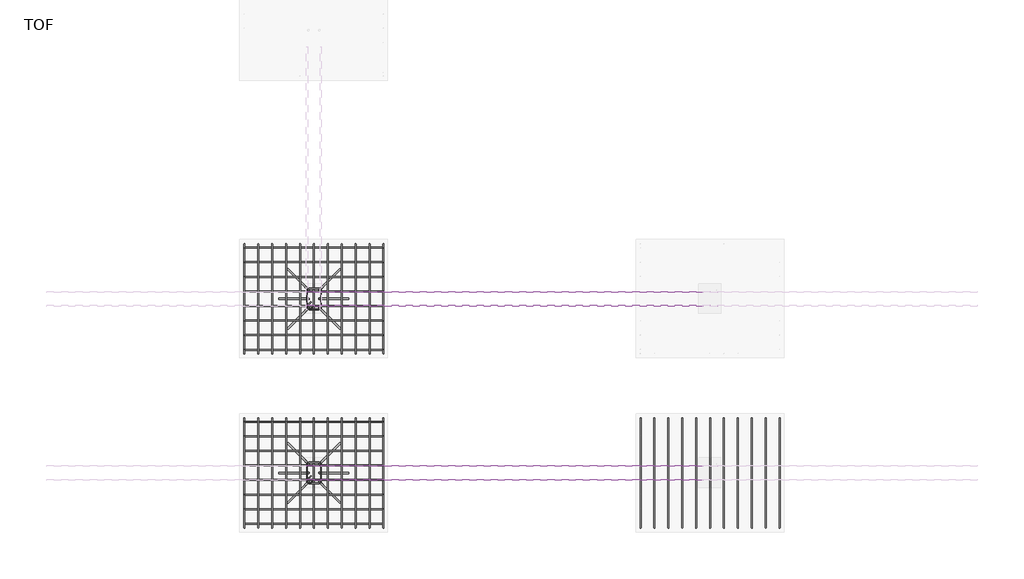
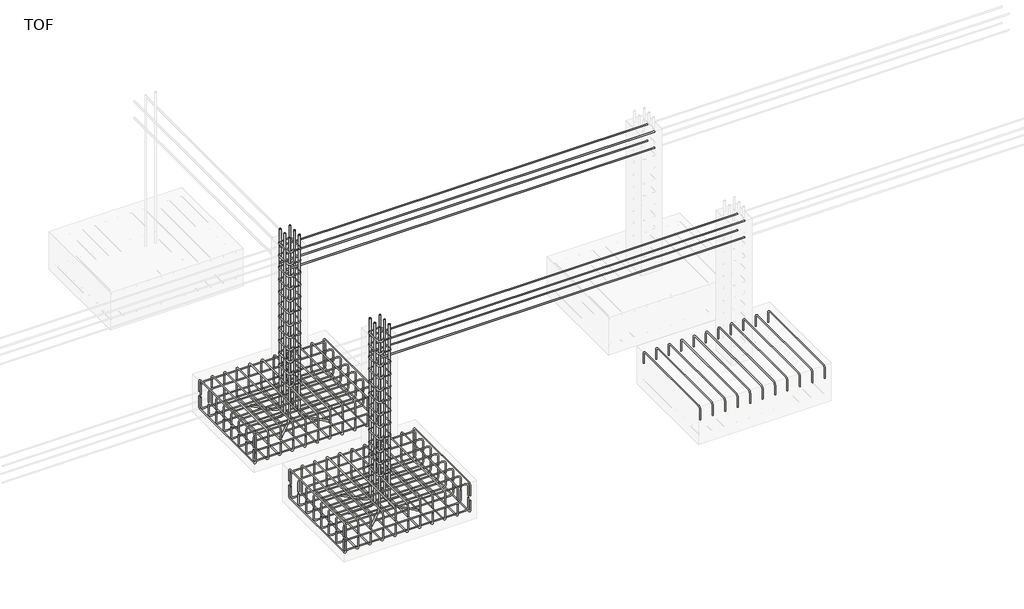
# One storey, part 4 of 10: 31 reinforcing bars.
"""IFC4 building model written with IfcOpenShell, lengths in millimetres."""

from ifc_helpers import new_model, si_unit, point, frame, origin, place, context, project, spatial, polyline, circle_curve, trimmed, segment, composite_curve, source, transform, mapped, element, save
from ifc_brep_helpers import swept_disk

model = new_model("IFC4")

# Units and contexts
model_context = context("Model", 3, world=origin())
ifc_project = project(units=[si_unit("LENGTHUNIT", "METRE", prefix="MILLI")], contexts=[model_context])

# Site, building, storey
site = spatial("IfcSite", under=ifc_project)
building = spatial("IfcBuilding", under=site)
storey = spatial("IfcBuildingStorey", under=building, Name="TOF", Elevation=-1828.8)

# Reinforcing bars
placement = place(None, origin())
reinforcing_bar_shape = source(origin(), model_context, "Body", "SolidModel", [
    swept_disk(composite_curve([segment(polyline([(2315.2782143, -14539.6267376, -2018.8), (2315.2782143, -14539.6267376, -1908.8)]), True, "CONTINUOUS"), segment(trimmed(circle_curve(frame((2315.2782143, -14574.6267376, -1908.8), z_axis=(1.0, 0.0, 0.0), x_axis=(0.0, 35.0, 0.0)), 35.0), [point((2315.2782143, -14539.6267376, -1908.8))], [point((2315.2782143, -14574.6267376, -1873.8))], True, "CARTESIAN"), True, "CONTINUOUS"), segment(polyline([(2315.2782143, -14574.6267376, -1873.8), (2315.2782143, -15614.6267376, -1873.8)]), True, "CONTINUOUS"), segment(trimmed(circle_curve(frame((2315.2782143, -15614.6267376, -1908.8), z_axis=(1.0, 0.0, 0.0), x_axis=(0.0, 0.0, 35.0)), 35.0), [point((2315.2782143, -15614.6267376, -1873.8))], [point((2315.2782143, -15649.6267376, -1908.8))], True, "CARTESIAN"), True, "CONTINUOUS"), segment(polyline([(2315.2782143, -15649.6267376, -1908.8), (2315.2782143, -15649.6267376, -2018.8)]), True, "CONTINUOUS")], self_intersect=False), 5.0),
])
element("IfcReinforcingBar", 1, at=placement, inside=storey, context=model_context, shape_type="MappedRepresentation", body=[
    mapped(reinforcing_bar_shape, transform((0.0, 0.0, 0.0), x_axis=(1.0, 0.0, 0.0), y_axis=(0.0, 1.0, 0.0), z_axis=(0.0, 0.0, 1.0))),
    mapped(reinforcing_bar_shape, transform((-141.0, 0.0, 0.0), x_axis=(1.0, 0.0, 0.0), y_axis=(0.0, 1.0, 0.0), z_axis=(0.0, 0.0, 1.0))),
    mapped(reinforcing_bar_shape, transform((-282.0, 0.0, 0.0), x_axis=(1.0, 0.0, 0.0), y_axis=(0.0, 1.0, 0.0), z_axis=(0.0, 0.0, 1.0))),
    mapped(reinforcing_bar_shape, transform((-423.0, 0.0, 0.0), x_axis=(1.0, 0.0, 0.0), y_axis=(0.0, 1.0, 0.0), z_axis=(0.0, 0.0, 1.0))),
    mapped(reinforcing_bar_shape, transform((-564.0, 0.0, 0.0), x_axis=(1.0, 0.0, 0.0), y_axis=(0.0, 1.0, 0.0), z_axis=(0.0, 0.0, 1.0))),
    mapped(reinforcing_bar_shape, transform((-705.0, 0.0, 0.0), x_axis=(1.0, 0.0, 0.0), y_axis=(0.0, 1.0, 0.0), z_axis=(0.0, 0.0, 1.0))),
    mapped(reinforcing_bar_shape, transform((-846.0, 0.0, 0.0), x_axis=(1.0, 0.0, 0.0), y_axis=(0.0, 1.0, 0.0), z_axis=(0.0, 0.0, 1.0))),
    mapped(reinforcing_bar_shape, transform((-987.0, 0.0, 0.0), x_axis=(1.0, 0.0, 0.0), y_axis=(0.0, 1.0, 0.0), z_axis=(0.0, 0.0, 1.0))),
    mapped(reinforcing_bar_shape, transform((-1128.0, 0.0, 0.0), x_axis=(1.0, 0.0, 0.0), y_axis=(0.0, 1.0, 0.0), z_axis=(0.0, 0.0, 1.0))),
    mapped(reinforcing_bar_shape, transform((-1269.0, 0.0, 0.0), x_axis=(1.0, 0.0, 0.0), y_axis=(0.0, 1.0, 0.0), z_axis=(0.0, 0.0, 1.0))),
    mapped(reinforcing_bar_shape, transform((-1410.0, 0.0, 0.0), x_axis=(1.0, 0.0, 0.0), y_axis=(0.0, 1.0, 0.0), z_axis=(0.0, 0.0, 1.0))),
])
reinforcing_bar_2_shape = source(origin(), model_context, "Body", "SolidModel", [
    swept_disk(composite_curve([segment(polyline([(2315.2782143, -15649.6267376, -2077.5233378), (2315.2782143, -15649.6267376, -2187.5233378)]), True, "CONTINUOUS"), segment(trimmed(circle_curve(frame((2315.2782143, -15614.6267376, -2187.5233378), z_axis=(1.0, 0.0, 0.0), x_axis=(0.0, -35.0, 0.0)), 35.0), [point((2315.2782143, -15649.6267376, -2187.5233378))], [point((2315.2782143, -15614.6267376, -2222.5233378))], True, "CARTESIAN"), True, "CONTINUOUS"), segment(polyline([(2315.2782143, -15614.6267376, -2222.5233378), (2315.2782143, -14574.6267376, -2222.5233378)]), True, "CONTINUOUS"), segment(trimmed(circle_curve(frame((2315.2782143, -14574.6267376, -2187.5233378), z_axis=(1.0, 0.0, 0.0), x_axis=(0.0, 0.0, -35.0)), 35.0), [point((2315.2782143, -14574.6267376, -2222.5233378))], [point((2315.2782143, -14539.6267376, -2187.5233378))], True, "CARTESIAN"), True, "CONTINUOUS"), segment(polyline([(2315.2782143, -14539.6267376, -2187.5233378), (2315.2782143, -14539.6267376, -2077.5233378)]), True, "CONTINUOUS")], self_intersect=False), 5.0),
])
element("IfcReinforcingBar", 2, at=placement, inside=storey, context=model_context, shape_type="MappedRepresentation", body=[
    mapped(reinforcing_bar_2_shape, transform((0.0, 0.0, 0.0), x_axis=(1.0, 0.0, 0.0), y_axis=(0.0, 1.0, 0.0), z_axis=(0.0, 0.0, 1.0))),
    mapped(reinforcing_bar_2_shape, transform((-141.0, 0.0, 0.0), x_axis=(1.0, 0.0, 0.0), y_axis=(0.0, 1.0, 0.0), z_axis=(0.0, 0.0, 1.0))),
    mapped(reinforcing_bar_2_shape, transform((-282.0, 0.0, 0.0), x_axis=(1.0, 0.0, 0.0), y_axis=(0.0, 1.0, 0.0), z_axis=(0.0, 0.0, 1.0))),
    mapped(reinforcing_bar_2_shape, transform((-423.0, 0.0, 0.0), x_axis=(1.0, 0.0, 0.0), y_axis=(0.0, 1.0, 0.0), z_axis=(0.0, 0.0, 1.0))),
    mapped(reinforcing_bar_2_shape, transform((-564.0, 0.0, 0.0), x_axis=(1.0, 0.0, 0.0), y_axis=(0.0, 1.0, 0.0), z_axis=(0.0, 0.0, 1.0))),
    mapped(reinforcing_bar_2_shape, transform((-705.0, 0.0, 0.0), x_axis=(1.0, 0.0, 0.0), y_axis=(0.0, 1.0, 0.0), z_axis=(0.0, 0.0, 1.0))),
    mapped(reinforcing_bar_2_shape, transform((-846.0, 0.0, 0.0), x_axis=(1.0, 0.0, 0.0), y_axis=(0.0, 1.0, 0.0), z_axis=(0.0, 0.0, 1.0))),
    mapped(reinforcing_bar_2_shape, transform((-987.0, 0.0, 0.0), x_axis=(1.0, 0.0, 0.0), y_axis=(0.0, 1.0, 0.0), z_axis=(0.0, 0.0, 1.0))),
    mapped(reinforcing_bar_2_shape, transform((-1128.0, 0.0, 0.0), x_axis=(1.0, 0.0, 0.0), y_axis=(0.0, 1.0, 0.0), z_axis=(0.0, 0.0, 1.0))),
    mapped(reinforcing_bar_2_shape, transform((-1269.0, 0.0, 0.0), x_axis=(1.0, 0.0, 0.0), y_axis=(0.0, 1.0, 0.0), z_axis=(0.0, 0.0, 1.0))),
    mapped(reinforcing_bar_2_shape, transform((-1410.0, 0.0, 0.0), x_axis=(1.0, 0.0, 0.0), y_axis=(0.0, 1.0, 0.0), z_axis=(0.0, 0.0, 1.0))),
])
reinforcing_bar_3_shape = source(origin(), model_context, "Body", "SolidModel", [
    swept_disk(composite_curve([segment(polyline([(2315.2782143, -14574.6861459, -2066.1776706), (2315.2782143, -14574.6861459, -2176.1776706)]), True, "CONTINUOUS"), segment(trimmed(circle_curve(frame((2280.2782143, -14574.6861459, -2176.1776706), z_axis=(0.0, 1.0, 0.0), x_axis=(35.0, 0.0, 0.0)), 35.0), [point((2315.2782143, -14574.6861459, -2176.1776706))], [point((2280.2782143, -14574.6861459, -2211.1776706))], True, "CARTESIAN"), True, "CONTINUOUS"), segment(polyline([(2280.2782143, -14574.6861459, -2211.1776706), (940.2782143, -14574.6861459, -2211.1776706)]), True, "CONTINUOUS"), segment(trimmed(circle_curve(frame((940.2782143, -14574.6861459, -2176.1776706), z_axis=(0.0, 1.0, 0.0), x_axis=(0.0, 0.0, -35.0)), 35.0), [point((940.2782143, -14574.6861459, -2211.1776706))], [point((905.2782143, -14574.6861459, -2176.1776706))], True, "CARTESIAN"), True, "CONTINUOUS"), segment(polyline([(905.2782143, -14574.6861459, -2176.1776706), (905.2782143, -14574.6861459, -2066.1776706)]), True, "CONTINUOUS")], self_intersect=False), 5.0),
])
element("IfcReinforcingBar", 3, at=placement, inside=storey, context=model_context, shape_type="MappedRepresentation", body=[
    mapped(reinforcing_bar_3_shape, transform((0.0, 0.0, 0.0), x_axis=(1.0, 0.0, 0.0), y_axis=(0.0, 1.0, 0.0), z_axis=(0.0, 0.0, 1.0))),
    mapped(reinforcing_bar_3_shape, transform((0.0, -148.0321606, 0.0), x_axis=(1.0, 0.0, 0.0), y_axis=(0.0, 1.0, 0.0), z_axis=(0.0, 0.0, 1.0))),
    mapped(reinforcing_bar_3_shape, transform((0.0, -296.0643211, 0.0), x_axis=(1.0, 0.0, 0.0), y_axis=(0.0, 1.0, 0.0), z_axis=(0.0, 0.0, 1.0))),
    mapped(reinforcing_bar_3_shape, transform((0.0, -444.0964817, 0.0), x_axis=(1.0, 0.0, 0.0), y_axis=(0.0, 1.0, 0.0), z_axis=(0.0, 0.0, 1.0))),
    mapped(reinforcing_bar_3_shape, transform((0.0, -592.1286423, 0.0), x_axis=(1.0, 0.0, 0.0), y_axis=(0.0, 1.0, 0.0), z_axis=(0.0, 0.0, 1.0))),
    mapped(reinforcing_bar_3_shape, transform((0.0, -740.1608029, 0.0), x_axis=(1.0, 0.0, 0.0), y_axis=(0.0, 1.0, 0.0), z_axis=(0.0, 0.0, 1.0))),
    mapped(reinforcing_bar_3_shape, transform((0.0, -888.1929634, 0.0), x_axis=(1.0, 0.0, 0.0), y_axis=(0.0, 1.0, 0.0), z_axis=(0.0, 0.0, 1.0))),
    mapped(reinforcing_bar_3_shape, transform((0.0, -1036.225124, 0.0), x_axis=(1.0, 0.0, 0.0), y_axis=(0.0, 1.0, 0.0), z_axis=(0.0, 0.0, 1.0))),
])
reinforcing_bar_4_shape = source(origin(), model_context, "Body", "SolidModel", [
    swept_disk(composite_curve([segment(polyline([(2315.2782143, -15610.9112699, -2039.256778), (2315.2782143, -15610.9112699, -1929.256778)]), True, "CONTINUOUS"), segment(trimmed(circle_curve(frame((2280.2782143, -15610.9112699, -1929.256778), z_axis=(0.0, -1.0, 0.0), x_axis=(35.0, 0.0, 0.0)), 35.0), [point((2315.2782143, -15610.9112699, -1929.256778))], [point((2280.2782143, -15610.9112699, -1894.256778))], True, "CARTESIAN"), True, "CONTINUOUS"), segment(polyline([(2280.2782143, -15610.9112699, -1894.256778), (940.2782143, -15610.9112699, -1894.256778)]), True, "CONTINUOUS"), segment(trimmed(circle_curve(frame((940.2782143, -15610.9112699, -1929.256778), z_axis=(0.0, -1.0, 0.0), x_axis=(0.0, 0.0, 35.0)), 35.0), [point((940.2782143, -15610.9112699, -1894.256778))], [point((905.2782143, -15610.9112699, -1929.256778))], True, "CARTESIAN"), True, "CONTINUOUS"), segment(polyline([(905.2782143, -15610.9112699, -1929.256778), (905.2782143, -15610.9112699, -2039.256778)]), True, "CONTINUOUS")], self_intersect=False), 5.0),
])
element("IfcReinforcingBar", 4, at=placement, inside=storey, context=model_context, shape_type="MappedRepresentation", body=[
    mapped(reinforcing_bar_4_shape, transform((0.0, 0.0, 0.0), x_axis=(1.0, 0.0, 0.0), y_axis=(0.0, 1.0, 0.0), z_axis=(0.0, 0.0, 1.0))),
    mapped(reinforcing_bar_4_shape, transform((0.0, 148.0321606, 0.0), x_axis=(1.0, 0.0, 0.0), y_axis=(0.0, 1.0, 0.0), z_axis=(0.0, 0.0, 1.0))),
    mapped(reinforcing_bar_4_shape, transform((0.0, 296.0643211, 0.0), x_axis=(1.0, 0.0, 0.0), y_axis=(0.0, 1.0, 0.0), z_axis=(0.0, 0.0, 1.0))),
    mapped(reinforcing_bar_4_shape, transform((0.0, 444.0964817, 0.0), x_axis=(1.0, 0.0, 0.0), y_axis=(0.0, 1.0, 0.0), z_axis=(0.0, 0.0, 1.0))),
    mapped(reinforcing_bar_4_shape, transform((0.0, 592.1286423, 0.0), x_axis=(1.0, 0.0, 0.0), y_axis=(0.0, 1.0, 0.0), z_axis=(0.0, 0.0, 1.0))),
    mapped(reinforcing_bar_4_shape, transform((0.0, 740.1608029, 0.0), x_axis=(1.0, 0.0, 0.0), y_axis=(0.0, 1.0, 0.0), z_axis=(0.0, 0.0, 1.0))),
    mapped(reinforcing_bar_4_shape, transform((0.0, 888.1929634, 0.0), x_axis=(1.0, 0.0, 0.0), y_axis=(0.0, 1.0, 0.0), z_axis=(0.0, 0.0, 1.0))),
    mapped(reinforcing_bar_4_shape, transform((0.0, 1036.225124, 0.0), x_axis=(1.0, 0.0, 0.0), y_axis=(0.0, 1.0, 0.0), z_axis=(0.0, 0.0, 1.0))),
])
reinforcing_bar_5_shape = source(origin(), model_context, "Body", "SolidModel", [
    swept_disk(composite_curve([segment(polyline([(6330.2782143, -14539.6267376, -2018.8), (6330.2782143, -14539.6267376, -1908.8)]), True, "CONTINUOUS"), segment(trimmed(circle_curve(frame((6330.2782143, -14574.6267376, -1908.8), z_axis=(1.0, 0.0, 0.0), x_axis=(0.0, 35.0, 0.0)), 35.0), [point((6330.2782143, -14539.6267376, -1908.8))], [point((6330.2782143, -14574.6267376, -1873.8))], True, "CARTESIAN"), True, "CONTINUOUS"), segment(polyline([(6330.2782143, -14574.6267376, -1873.8), (6330.2782143, -15614.6267376, -1873.8)]), True, "CONTINUOUS"), segment(trimmed(circle_curve(frame((6330.2782143, -15614.6267376, -1908.8), z_axis=(1.0, 0.0, 0.0), x_axis=(0.0, 0.0, 35.0)), 35.0), [point((6330.2782143, -15614.6267376, -1873.8))], [point((6330.2782143, -15649.6267376, -1908.8))], True, "CARTESIAN"), True, "CONTINUOUS"), segment(polyline([(6330.2782143, -15649.6267376, -1908.8), (6330.2782143, -15649.6267376, -2018.8)]), True, "CONTINUOUS")], self_intersect=False), 5.0),
])
element("IfcReinforcingBar", 5, at=placement, inside=storey, context=model_context, shape_type="MappedRepresentation", body=[
    mapped(reinforcing_bar_5_shape, transform((0.0, 0.0, 0.0), x_axis=(1.0, 0.0, 0.0), y_axis=(0.0, 1.0, 0.0), z_axis=(0.0, 0.0, 1.0))),
    mapped(reinforcing_bar_5_shape, transform((-141.0, 0.0, 0.0), x_axis=(1.0, 0.0, 0.0), y_axis=(0.0, 1.0, 0.0), z_axis=(0.0, 0.0, 1.0))),
    mapped(reinforcing_bar_5_shape, transform((-282.0, 0.0, 0.0), x_axis=(1.0, 0.0, 0.0), y_axis=(0.0, 1.0, 0.0), z_axis=(0.0, 0.0, 1.0))),
    mapped(reinforcing_bar_5_shape, transform((-423.0, 0.0, 0.0), x_axis=(1.0, 0.0, 0.0), y_axis=(0.0, 1.0, 0.0), z_axis=(0.0, 0.0, 1.0))),
    mapped(reinforcing_bar_5_shape, transform((-564.0, 0.0, 0.0), x_axis=(1.0, 0.0, 0.0), y_axis=(0.0, 1.0, 0.0), z_axis=(0.0, 0.0, 1.0))),
    mapped(reinforcing_bar_5_shape, transform((-705.0, 0.0, 0.0), x_axis=(1.0, 0.0, 0.0), y_axis=(0.0, 1.0, 0.0), z_axis=(0.0, 0.0, 1.0))),
    mapped(reinforcing_bar_5_shape, transform((-846.0, 0.0, 0.0), x_axis=(1.0, 0.0, 0.0), y_axis=(0.0, 1.0, 0.0), z_axis=(0.0, 0.0, 1.0))),
    mapped(reinforcing_bar_5_shape, transform((-987.0, 0.0, 0.0), x_axis=(1.0, 0.0, 0.0), y_axis=(0.0, 1.0, 0.0), z_axis=(0.0, 0.0, 1.0))),
    mapped(reinforcing_bar_5_shape, transform((-1128.0, 0.0, 0.0), x_axis=(1.0, 0.0, 0.0), y_axis=(0.0, 1.0, 0.0), z_axis=(0.0, 0.0, 1.0))),
    mapped(reinforcing_bar_5_shape, transform((-1269.0, 0.0, 0.0), x_axis=(1.0, 0.0, 0.0), y_axis=(0.0, 1.0, 0.0), z_axis=(0.0, 0.0, 1.0))),
    mapped(reinforcing_bar_5_shape, transform((-1410.0, 0.0, 0.0), x_axis=(1.0, 0.0, 0.0), y_axis=(0.0, 1.0, 0.0), z_axis=(0.0, 0.0, 1.0))),
])
reinforcing_bar_6_shape = source(origin(), model_context, "Body", "SolidModel", [
    swept_disk(composite_curve([segment(polyline([(2315.2782143, -12774.6267376, -2018.8), (2315.2782143, -12774.6267376, -1908.8)]), True, "CONTINUOUS"), segment(trimmed(circle_curve(frame((2315.2782143, -12809.6267376, -1908.8), z_axis=(1.0, 0.0, 0.0), x_axis=(0.0, 35.0, 0.0)), 35.0), [point((2315.2782143, -12774.6267376, -1908.8))], [point((2315.2782143, -12809.6267376, -1873.8))], True, "CARTESIAN"), True, "CONTINUOUS"), segment(polyline([(2315.2782143, -12809.6267376, -1873.8), (2315.2782143, -13849.6267376, -1873.8)]), True, "CONTINUOUS"), segment(trimmed(circle_curve(frame((2315.2782143, -13849.6267376, -1908.8), z_axis=(1.0, 0.0, 0.0), x_axis=(0.0, 0.0, 35.0)), 35.0), [point((2315.2782143, -13849.6267376, -1873.8))], [point((2315.2782143, -13884.6267376, -1908.8))], True, "CARTESIAN"), True, "CONTINUOUS"), segment(polyline([(2315.2782143, -13884.6267376, -1908.8), (2315.2782143, -13884.6267376, -2018.8)]), True, "CONTINUOUS")], self_intersect=False), 5.0),
])
element("IfcReinforcingBar", 6, at=placement, inside=storey, context=model_context, shape_type="MappedRepresentation", body=[
    mapped(reinforcing_bar_6_shape, transform((0.0, 0.0, 0.0), x_axis=(1.0, 0.0, 0.0), y_axis=(0.0, 1.0, 0.0), z_axis=(0.0, 0.0, 1.0))),
    mapped(reinforcing_bar_6_shape, transform((-141.0, 0.0, 0.0), x_axis=(1.0, 0.0, 0.0), y_axis=(0.0, 1.0, 0.0), z_axis=(0.0, 0.0, 1.0))),
    mapped(reinforcing_bar_6_shape, transform((-282.0, 0.0, 0.0), x_axis=(1.0, 0.0, 0.0), y_axis=(0.0, 1.0, 0.0), z_axis=(0.0, 0.0, 1.0))),
    mapped(reinforcing_bar_6_shape, transform((-423.0, 0.0, 0.0), x_axis=(1.0, 0.0, 0.0), y_axis=(0.0, 1.0, 0.0), z_axis=(0.0, 0.0, 1.0))),
    mapped(reinforcing_bar_6_shape, transform((-564.0, 0.0, 0.0), x_axis=(1.0, 0.0, 0.0), y_axis=(0.0, 1.0, 0.0), z_axis=(0.0, 0.0, 1.0))),
    mapped(reinforcing_bar_6_shape, transform((-705.0, 0.0, 0.0), x_axis=(1.0, 0.0, 0.0), y_axis=(0.0, 1.0, 0.0), z_axis=(0.0, 0.0, 1.0))),
    mapped(reinforcing_bar_6_shape, transform((-846.0, 0.0, 0.0), x_axis=(1.0, 0.0, 0.0), y_axis=(0.0, 1.0, 0.0), z_axis=(0.0, 0.0, 1.0))),
    mapped(reinforcing_bar_6_shape, transform((-987.0, 0.0, 0.0), x_axis=(1.0, 0.0, 0.0), y_axis=(0.0, 1.0, 0.0), z_axis=(0.0, 0.0, 1.0))),
    mapped(reinforcing_bar_6_shape, transform((-1128.0, 0.0, 0.0), x_axis=(1.0, 0.0, 0.0), y_axis=(0.0, 1.0, 0.0), z_axis=(0.0, 0.0, 1.0))),
    mapped(reinforcing_bar_6_shape, transform((-1269.0, 0.0, 0.0), x_axis=(1.0, 0.0, 0.0), y_axis=(0.0, 1.0, 0.0), z_axis=(0.0, 0.0, 1.0))),
    mapped(reinforcing_bar_6_shape, transform((-1410.0, 0.0, 0.0), x_axis=(1.0, 0.0, 0.0), y_axis=(0.0, 1.0, 0.0), z_axis=(0.0, 0.0, 1.0))),
])
reinforcing_bar_7_shape = source(origin(), model_context, "Body", "SolidModel", [
    swept_disk(composite_curve([segment(polyline([(2315.2782143, -13884.6267376, -2077.5233378), (2315.2782143, -13884.6267376, -2187.5233378)]), True, "CONTINUOUS"), segment(trimmed(circle_curve(frame((2315.2782143, -13849.6267376, -2187.5233378), z_axis=(1.0, 0.0, 0.0), x_axis=(0.0, -35.0, 0.0)), 35.0), [point((2315.2782143, -13884.6267376, -2187.5233378))], [point((2315.2782143, -13849.6267376, -2222.5233378))], True, "CARTESIAN"), True, "CONTINUOUS"), segment(polyline([(2315.2782143, -13849.6267376, -2222.5233378), (2315.2782143, -12809.6267376, -2222.5233378)]), True, "CONTINUOUS"), segment(trimmed(circle_curve(frame((2315.2782143, -12809.6267376, -2187.5233378), z_axis=(1.0, 0.0, 0.0), x_axis=(0.0, 0.0, -35.0)), 35.0), [point((2315.2782143, -12809.6267376, -2222.5233378))], [point((2315.2782143, -12774.6267376, -2187.5233378))], True, "CARTESIAN"), True, "CONTINUOUS"), segment(polyline([(2315.2782143, -12774.6267376, -2187.5233378), (2315.2782143, -12774.6267376, -2077.5233378)]), True, "CONTINUOUS")], self_intersect=False), 5.0),
])
element("IfcReinforcingBar", 7, at=placement, inside=storey, context=model_context, shape_type="MappedRepresentation", body=[
    mapped(reinforcing_bar_7_shape, transform((0.0, 0.0, 0.0), x_axis=(1.0, 0.0, 0.0), y_axis=(0.0, 1.0, 0.0), z_axis=(0.0, 0.0, 1.0))),
    mapped(reinforcing_bar_7_shape, transform((-141.0, 0.0, 0.0), x_axis=(1.0, 0.0, 0.0), y_axis=(0.0, 1.0, 0.0), z_axis=(0.0, 0.0, 1.0))),
    mapped(reinforcing_bar_7_shape, transform((-282.0, 0.0, 0.0), x_axis=(1.0, 0.0, 0.0), y_axis=(0.0, 1.0, 0.0), z_axis=(0.0, 0.0, 1.0))),
    mapped(reinforcing_bar_7_shape, transform((-423.0, 0.0, 0.0), x_axis=(1.0, 0.0, 0.0), y_axis=(0.0, 1.0, 0.0), z_axis=(0.0, 0.0, 1.0))),
    mapped(reinforcing_bar_7_shape, transform((-564.0, 0.0, 0.0), x_axis=(1.0, 0.0, 0.0), y_axis=(0.0, 1.0, 0.0), z_axis=(0.0, 0.0, 1.0))),
    mapped(reinforcing_bar_7_shape, transform((-705.0, 0.0, 0.0), x_axis=(1.0, 0.0, 0.0), y_axis=(0.0, 1.0, 0.0), z_axis=(0.0, 0.0, 1.0))),
    mapped(reinforcing_bar_7_shape, transform((-846.0, 0.0, 0.0), x_axis=(1.0, 0.0, 0.0), y_axis=(0.0, 1.0, 0.0), z_axis=(0.0, 0.0, 1.0))),
    mapped(reinforcing_bar_7_shape, transform((-987.0, 0.0, 0.0), x_axis=(1.0, 0.0, 0.0), y_axis=(0.0, 1.0, 0.0), z_axis=(0.0, 0.0, 1.0))),
    mapped(reinforcing_bar_7_shape, transform((-1128.0, 0.0, 0.0), x_axis=(1.0, 0.0, 0.0), y_axis=(0.0, 1.0, 0.0), z_axis=(0.0, 0.0, 1.0))),
    mapped(reinforcing_bar_7_shape, transform((-1269.0, 0.0, 0.0), x_axis=(1.0, 0.0, 0.0), y_axis=(0.0, 1.0, 0.0), z_axis=(0.0, 0.0, 1.0))),
    mapped(reinforcing_bar_7_shape, transform((-1410.0, 0.0, 0.0), x_axis=(1.0, 0.0, 0.0), y_axis=(0.0, 1.0, 0.0), z_axis=(0.0, 0.0, 1.0))),
])
reinforcing_bar_8_shape = source(origin(), model_context, "Body", "SolidModel", [
    swept_disk(composite_curve([segment(polyline([(2315.2782143, -12809.6861459, -2066.1776706), (2315.2782143, -12809.6861459, -2176.1776706)]), True, "CONTINUOUS"), segment(trimmed(circle_curve(frame((2280.2782143, -12809.6861459, -2176.1776706), z_axis=(0.0, 1.0, 0.0), x_axis=(35.0, 0.0, 0.0)), 35.0), [point((2315.2782143, -12809.6861459, -2176.1776706))], [point((2280.2782143, -12809.6861459, -2211.1776706))], True, "CARTESIAN"), True, "CONTINUOUS"), segment(polyline([(2280.2782143, -12809.6861459, -2211.1776706), (940.2782143, -12809.6861459, -2211.1776706)]), True, "CONTINUOUS"), segment(trimmed(circle_curve(frame((940.2782143, -12809.6861459, -2176.1776706), z_axis=(0.0, 1.0, 0.0), x_axis=(0.0, 0.0, -35.0)), 35.0), [point((940.2782143, -12809.6861459, -2211.1776706))], [point((905.2782143, -12809.6861459, -2176.1776706))], True, "CARTESIAN"), True, "CONTINUOUS"), segment(polyline([(905.2782143, -12809.6861459, -2176.1776706), (905.2782143, -12809.6861459, -2066.1776706)]), True, "CONTINUOUS")], self_intersect=False), 5.0),
])
element("IfcReinforcingBar", 8, at=placement, inside=storey, context=model_context, shape_type="MappedRepresentation", body=[
    mapped(reinforcing_bar_8_shape, transform((0.0, 0.0, 0.0), x_axis=(1.0, 0.0, 0.0), y_axis=(0.0, 1.0, 0.0), z_axis=(0.0, 0.0, 1.0))),
    mapped(reinforcing_bar_8_shape, transform((0.0, -148.0321606, 0.0), x_axis=(1.0, 0.0, 0.0), y_axis=(0.0, 1.0, 0.0), z_axis=(0.0, 0.0, 1.0))),
    mapped(reinforcing_bar_8_shape, transform((0.0, -296.0643211, 0.0), x_axis=(1.0, 0.0, 0.0), y_axis=(0.0, 1.0, 0.0), z_axis=(0.0, 0.0, 1.0))),
    mapped(reinforcing_bar_8_shape, transform((0.0, -444.0964817, 0.0), x_axis=(1.0, 0.0, 0.0), y_axis=(0.0, 1.0, 0.0), z_axis=(0.0, 0.0, 1.0))),
    mapped(reinforcing_bar_8_shape, transform((0.0, -592.1286423, 0.0), x_axis=(1.0, 0.0, 0.0), y_axis=(0.0, 1.0, 0.0), z_axis=(0.0, 0.0, 1.0))),
    mapped(reinforcing_bar_8_shape, transform((0.0, -740.1608029, 0.0), x_axis=(1.0, 0.0, 0.0), y_axis=(0.0, 1.0, 0.0), z_axis=(0.0, 0.0, 1.0))),
    mapped(reinforcing_bar_8_shape, transform((0.0, -888.1929634, 0.0), x_axis=(1.0, 0.0, 0.0), y_axis=(0.0, 1.0, 0.0), z_axis=(0.0, 0.0, 1.0))),
    mapped(reinforcing_bar_8_shape, transform((0.0, -1036.225124, 0.0), x_axis=(1.0, 0.0, 0.0), y_axis=(0.0, 1.0, 0.0), z_axis=(0.0, 0.0, 1.0))),
])
reinforcing_bar_9_shape = source(origin(), model_context, "Body", "SolidModel", [
    swept_disk(composite_curve([segment(polyline([(2315.2782143, -13845.9112699, -2039.256778), (2315.2782143, -13845.9112699, -1929.256778)]), True, "CONTINUOUS"), segment(trimmed(circle_curve(frame((2280.2782143, -13845.9112699, -1929.256778), z_axis=(0.0, -1.0, 0.0), x_axis=(35.0, 0.0, 0.0)), 35.0), [point((2315.2782143, -13845.9112699, -1929.256778))], [point((2280.2782143, -13845.9112699, -1894.256778))], True, "CARTESIAN"), True, "CONTINUOUS"), segment(polyline([(2280.2782143, -13845.9112699, -1894.256778), (940.2782143, -13845.9112699, -1894.256778)]), True, "CONTINUOUS"), segment(trimmed(circle_curve(frame((940.2782143, -13845.9112699, -1929.256778), z_axis=(0.0, -1.0, 0.0), x_axis=(0.0, 0.0, 35.0)), 35.0), [point((940.2782143, -13845.9112699, -1894.256778))], [point((905.2782143, -13845.9112699, -1929.256778))], True, "CARTESIAN"), True, "CONTINUOUS"), segment(polyline([(905.2782143, -13845.9112699, -1929.256778), (905.2782143, -13845.9112699, -2039.256778)]), True, "CONTINUOUS")], self_intersect=False), 5.0),
])
element("IfcReinforcingBar", 9, at=placement, inside=storey, context=model_context, shape_type="MappedRepresentation", body=[
    mapped(reinforcing_bar_9_shape, transform((0.0, 0.0, 0.0), x_axis=(1.0, 0.0, 0.0), y_axis=(0.0, 1.0, 0.0), z_axis=(0.0, 0.0, 1.0))),
    mapped(reinforcing_bar_9_shape, transform((0.0, 148.0321606, 0.0), x_axis=(1.0, 0.0, 0.0), y_axis=(0.0, 1.0, 0.0), z_axis=(0.0, 0.0, 1.0))),
    mapped(reinforcing_bar_9_shape, transform((0.0, 296.0643211, 0.0), x_axis=(1.0, 0.0, 0.0), y_axis=(0.0, 1.0, 0.0), z_axis=(0.0, 0.0, 1.0))),
    mapped(reinforcing_bar_9_shape, transform((0.0, 444.0964817, 0.0), x_axis=(1.0, 0.0, 0.0), y_axis=(0.0, 1.0, 0.0), z_axis=(0.0, 0.0, 1.0))),
    mapped(reinforcing_bar_9_shape, transform((0.0, 592.1286423, 0.0), x_axis=(1.0, 0.0, 0.0), y_axis=(0.0, 1.0, 0.0), z_axis=(0.0, 0.0, 1.0))),
    mapped(reinforcing_bar_9_shape, transform((0.0, 740.1608029, 0.0), x_axis=(1.0, 0.0, 0.0), y_axis=(0.0, 1.0, 0.0), z_axis=(0.0, 0.0, 1.0))),
    mapped(reinforcing_bar_9_shape, transform((0.0, 888.1929634, 0.0), x_axis=(1.0, 0.0, 0.0), y_axis=(0.0, 1.0, 0.0), z_axis=(0.0, 0.0, 1.0))),
    mapped(reinforcing_bar_9_shape, transform((0.0, 1036.225124, 0.0), x_axis=(1.0, 0.0, 0.0), y_axis=(0.0, 1.0, 0.0), z_axis=(0.0, 0.0, 1.0))),
])
reinforcing_bar_10_shape = source(origin(), model_context, "Body", "SolidModel", [
    swept_disk(composite_curve([segment(polyline([(1580.248777, -15125.7150493, -1784.8), (1546.3076515, -15159.6561748, -1784.8)]), True, "CONTINUOUS"), segment(trimmed(circle_curve(frame((1563.2782143, -15176.6267376, -1784.8), z_axis=(0.0, 0.0, 1.0), x_axis=(-16.970562799999925, 16.970562799999243, 0.0)), 24.0), [point((1546.3076515, -15159.6561748, -1784.8))], [point((1563.2782143, -15200.6267376, -1784.8))], True, "CARTESIAN"), True, "CONTINUOUS"), segment(polyline([(1563.2782143, -15200.6267376, -1784.8), (1657.2782143, -15200.6267376, -1784.8)]), True, "CONTINUOUS"), segment(trimmed(circle_curve(frame((1657.2782143, -15176.6267376, -1784.8), z_axis=(0.0, 0.0, 1.0), x_axis=(0.0, -24.0, 0.0)), 24.0), [point((1657.2782143, -15200.6267376, -1784.8))], [point((1681.2782143, -15176.6267376, -1784.8))], True, "CARTESIAN"), True, "CONTINUOUS"), segment(polyline([(1681.2782143, -15176.6267376, -1784.8), (1681.2782143, -15012.6267376, -1784.8)]), True, "CONTINUOUS"), segment(trimmed(circle_curve(frame((1657.3162115, -15012.6267376, -1786.149972), z_axis=(-0.05624883273897078, 0.0, 0.9984167811167355), x_axis=(23.962002799999937, 0.0, 1.3499719999999797)), 24.0), [point((1681.2782143, -15012.6267376, -1784.8))], [point((1657.3162115, -14988.6267376, -1786.149972))], True, "CARTESIAN"), True, "CONTINUOUS"), segment(polyline([(1657.3162115, -14988.6267376, -1786.149972), (1563.240217, -14988.6267376, -1791.450028)]), True, "CONTINUOUS"), segment(trimmed(circle_curve(frame((1563.240217, -15012.6267376, -1791.450028), z_axis=(-0.05624883273897078, 0.0, 0.9984167811167355), x_axis=(0.0, 24.0, 0.0)), 24.0), [point((1563.240217, -14988.6267376, -1791.450028))], [point((1539.2782143, -15012.6267376, -1792.8))], True, "CARTESIAN"), True, "CONTINUOUS"), segment(polyline([(1539.2782143, -15012.6267376, -1792.8), (1539.2782143, -15176.6267376, -1792.8)]), True, "CONTINUOUS"), segment(trimmed(circle_curve(frame((1563.2782143, -15176.6267376, -1792.8), z_axis=(0.0, 0.0, 1.0), x_axis=(-24.0, 0.0, 0.0)), 24.0), [point((1539.2782143, -15176.6267376, -1792.8))], [point((1580.248777, -15193.5973003, -1792.8))], True, "CARTESIAN"), True, "CONTINUOUS"), segment(polyline([(1580.248777, -15193.5973003, -1792.8), (1614.1899025, -15159.6561748, -1792.8)]), True, "CONTINUOUS")], self_intersect=False), 4.0),
])
element("IfcReinforcingBar", 10, at=placement, inside=storey, context=model_context, shape_type="MappedRepresentation", body=[
    mapped(reinforcing_bar_10_shape, transform((0.0, 0.0, 0.0), x_axis=(1.0, 0.0, 0.0), y_axis=(0.0, 1.0, 0.0), z_axis=(0.0, 0.0, 1.0))),
    mapped(reinforcing_bar_10_shape, transform((0.0, 0.0, 145.9395608), x_axis=(1.0, 0.0, 0.0), y_axis=(0.0, 1.0, 0.0), z_axis=(0.0, 0.0, 1.0))),
    mapped(reinforcing_bar_10_shape, transform((0.0, 0.0, 291.8791216), x_axis=(1.0, 0.0, 0.0), y_axis=(0.0, 1.0, 0.0), z_axis=(0.0, 0.0, 1.0))),
    mapped(reinforcing_bar_10_shape, transform((0.0, 0.0, 437.8186825), x_axis=(1.0, 0.0, 0.0), y_axis=(0.0, 1.0, 0.0), z_axis=(0.0, 0.0, 1.0))),
    mapped(reinforcing_bar_10_shape, transform((0.0, 0.0, 583.7582433), x_axis=(1.0, 0.0, 0.0), y_axis=(0.0, 1.0, 0.0), z_axis=(0.0, 0.0, 1.0))),
    mapped(reinforcing_bar_10_shape, transform((0.0, 0.0, 729.6978041), x_axis=(1.0, 0.0, 0.0), y_axis=(0.0, 1.0, 0.0), z_axis=(0.0, 0.0, 1.0))),
    mapped(reinforcing_bar_10_shape, transform((0.0, 0.0, 875.6373649), x_axis=(1.0, 0.0, 0.0), y_axis=(0.0, 1.0, 0.0), z_axis=(0.0, 0.0, 1.0))),
    mapped(reinforcing_bar_10_shape, transform((0.0, 0.0, 1021.5769258), x_axis=(1.0, 0.0, 0.0), y_axis=(0.0, 1.0, 0.0), z_axis=(0.0, 0.0, 1.0))),
    mapped(reinforcing_bar_10_shape, transform((0.0, 0.0, 1167.5164866), x_axis=(1.0, 0.0, 0.0), y_axis=(0.0, 1.0, 0.0), z_axis=(0.0, 0.0, 1.0))),
    mapped(reinforcing_bar_10_shape, transform((0.0, 0.0, 1313.4560474), x_axis=(1.0, 0.0, 0.0), y_axis=(0.0, 1.0, 0.0), z_axis=(0.0, 0.0, 1.0))),
    mapped(reinforcing_bar_10_shape, transform((0.0, 0.0, 1459.3956082), x_axis=(1.0, 0.0, 0.0), y_axis=(0.0, 1.0, 0.0), z_axis=(0.0, 0.0, 1.0))),
    mapped(reinforcing_bar_10_shape, transform((0.0, 0.0, 1605.3351691), x_axis=(1.0, 0.0, 0.0), y_axis=(0.0, 1.0, 0.0), z_axis=(0.0, 0.0, 1.0))),
])
element("IfcReinforcingBar", 11, at=placement, inside=storey, context=model_context, shape_type="SolidModel", body=[
    swept_disk(composite_curve([segment(polyline([(1665.884816, -15185.2333393, -20.0), (1665.884816, -15185.2333393, -2138.7824747)]), True, "CONTINUOUS"), segment(trimmed(circle_curve(frame((1705.1292424, -15224.4777657, -2138.7824747), z_axis=(-0.7071067811865545, -0.7071067811865406, 0.0), x_axis=(-39.244426400000066, 39.2444263999987, 0.0)), 55.5), [point((1665.884816, -15185.2333393, -2138.7824747))], [point((1705.1292424, -15224.4777657, -2194.2824747))], True, "CARTESIAN"), True, "CONTINUOUS"), segment(polyline([(1705.1292424, -15224.4777657, -2194.2824747), (1877.5083915, -15396.8569148, -2194.2824747)]), True, "CONTINUOUS")], self_intersect=False), 8.0),
])
element("IfcReinforcingBar", 12, at=placement, inside=storey, context=model_context, shape_type="SolidModel", body=[
    swept_disk(composite_curve([segment(polyline([(1665.934816, -15094.6267376, -20.0), (1665.934816, -15094.6267376, -2138.7824747)]), True, "CONTINUOUS"), segment(trimmed(circle_curve(frame((1721.434816, -15094.6267376, -2138.7824747), z_axis=(0.0, -1.0, 0.0), x_axis=(-55.5, 0.0, 0.0)), 55.5), [point((1665.934816, -15094.6267376, -2138.7824747))], [point((1721.434816, -15094.6267376, -2194.2824747))], True, "CARTESIAN"), True, "CONTINUOUS"), segment(polyline([(1721.434816, -15094.6267376, -2194.2824747), (1965.1657466, -15094.6267376, -2194.2824747)]), True, "CONTINUOUS")], self_intersect=False), 8.0),
])
element("IfcReinforcingBar", 13, at=placement, inside=storey, context=model_context, shape_type="SolidModel", body=[
    swept_disk(composite_curve([segment(polyline([(1665.884816, -15004.0201359, -20.0), (1665.884816, -15004.0201359, -2138.7824747)]), True, "CONTINUOUS"), segment(trimmed(circle_curve(frame((1705.1292424, -14964.7757095, -2138.7824747), z_axis=(0.7071067811865545, -0.7071067811865407, 0.0), x_axis=(-39.244426400000066, -39.24442640000052, 0.0)), 55.5), [point((1665.884816, -15004.0201359, -2138.7824747))], [point((1705.1292424, -14964.7757095, -2194.2824747))], True, "CARTESIAN"), True, "CONTINUOUS"), segment(polyline([(1705.1292424, -14964.7757095, -2194.2824747), (1877.5083915, -14792.3965603, -2194.2824747)]), True, "CONTINUOUS")], self_intersect=False), 8.0),
])
element("IfcReinforcingBar", 14, at=placement, inside=storey, context=model_context, shape_type="SolidModel", body=[
    swept_disk(composite_curve([segment(polyline([(1554.6716126, -15185.2333393, -20.0), (1554.6716126, -15185.2333393, -2138.7824747)]), True, "CONTINUOUS"), segment(trimmed(circle_curve(frame((1515.4271862, -15224.4777657, -2138.7824747), z_axis=(-0.7071067811865517, 0.7071067811865434, 0.0), x_axis=(39.24442639999984, 39.2444263999987, 0.0)), 55.5), [point((1554.6716126, -15185.2333393, -2138.7824747))], [point((1515.4271862, -15224.4777657, -2194.2824747))], True, "CARTESIAN"), True, "CONTINUOUS"), segment(polyline([(1515.4271862, -15224.4777657, -2194.2824747), (1343.048037, -15396.8569148, -2194.2824747)]), True, "CONTINUOUS")], self_intersect=False), 8.0),
])
element("IfcReinforcingBar", 15, at=placement, inside=storey, context=model_context, shape_type="SolidModel", body=[
    swept_disk(composite_curve([segment(polyline([(1554.6216126, -15094.6267376, -20.0), (1554.6216126, -15094.6267376, -2138.7824747)]), True, "CONTINUOUS"), segment(trimmed(circle_curve(frame((1499.1216126, -15094.6267376, -2138.7824747), z_axis=(0.0, 1.0, 0.0), x_axis=(55.5, 0.0, 0.0)), 55.5), [point((1554.6216126, -15094.6267376, -2138.7824747))], [point((1499.1216126, -15094.6267376, -2194.2824747))], True, "CARTESIAN"), True, "CONTINUOUS"), segment(polyline([(1499.1216126, -15094.6267376, -2194.2824747), (1255.3906819, -15094.6267376, -2194.2824747)]), True, "CONTINUOUS")], self_intersect=False), 8.0),
])
element("IfcReinforcingBar", 16, at=placement, inside=storey, context=model_context, shape_type="SolidModel", body=[
    swept_disk(composite_curve([segment(polyline([(1554.6716126, -15004.0201359, -20.0), (1554.6716126, -15004.0201359, -2138.7824747)]), True, "CONTINUOUS"), segment(trimmed(circle_curve(frame((1515.4271862, -14964.7757095, -2138.7824747), z_axis=(0.7071067811865572, 0.7071067811865379, 0.0), x_axis=(39.24442639999984, -39.24442640000052, 0.0)), 55.5), [point((1554.6716126, -15004.0201359, -2138.7824747))], [point((1515.4271862, -14964.7757095, -2194.2824747))], True, "CARTESIAN"), True, "CONTINUOUS"), segment(polyline([(1515.4271862, -14964.7757095, -2194.2824747), (1343.048037, -14792.3965603, -2194.2824747)]), True, "CONTINUOUS")], self_intersect=False), 8.0),
])
reinforcing_bar_11_shape = source(origin(), model_context, "Body", "SolidModel", [
    swept_disk(composite_curve([segment(polyline([(1580.248777, -13360.7150493, -1784.8), (1546.3076515, -13394.6561748, -1784.8)]), True, "CONTINUOUS"), segment(trimmed(circle_curve(frame((1563.2782143, -13411.6267376, -1784.8), z_axis=(0.0, 0.0, 1.0), x_axis=(-16.970562799999925, 16.970562799999243, 0.0)), 24.0), [point((1546.3076515, -13394.6561748, -1784.8))], [point((1563.2782143, -13435.6267376, -1784.8))], True, "CARTESIAN"), True, "CONTINUOUS"), segment(polyline([(1563.2782143, -13435.6267376, -1784.8), (1657.2782143, -13435.6267376, -1784.8)]), True, "CONTINUOUS"), segment(trimmed(circle_curve(frame((1657.2782143, -13411.6267376, -1784.8), z_axis=(0.0, 0.0, 1.0), x_axis=(0.0, -24.0, 0.0)), 24.0), [point((1657.2782143, -13435.6267376, -1784.8))], [point((1681.2782143, -13411.6267376, -1784.8))], True, "CARTESIAN"), True, "CONTINUOUS"), segment(polyline([(1681.2782143, -13411.6267376, -1784.8), (1681.2782143, -13247.6267376, -1784.8)]), True, "CONTINUOUS"), segment(trimmed(circle_curve(frame((1657.3162115, -13247.6267376, -1786.149972), z_axis=(-0.05624883273897078, 0.0, 0.9984167811167355), x_axis=(23.962002799999937, 0.0, 1.3499719999999797)), 24.0), [point((1681.2782143, -13247.6267376, -1784.8))], [point((1657.3162115, -13223.6267376, -1786.149972))], True, "CARTESIAN"), True, "CONTINUOUS"), segment(polyline([(1657.3162115, -13223.6267376, -1786.149972), (1563.240217, -13223.6267376, -1791.450028)]), True, "CONTINUOUS"), segment(trimmed(circle_curve(frame((1563.240217, -13247.6267376, -1791.450028), z_axis=(-0.05624883273897078, 0.0, 0.9984167811167355), x_axis=(0.0, 24.0, 0.0)), 24.0), [point((1563.240217, -13223.6267376, -1791.450028))], [point((1539.2782143, -13247.6267376, -1792.8))], True, "CARTESIAN"), True, "CONTINUOUS"), segment(polyline([(1539.2782143, -13247.6267376, -1792.8), (1539.2782143, -13411.6267376, -1792.8)]), True, "CONTINUOUS"), segment(trimmed(circle_curve(frame((1563.2782143, -13411.6267376, -1792.8), z_axis=(0.0, 0.0, 1.0), x_axis=(-24.0, 0.0, 0.0)), 24.0), [point((1539.2782143, -13411.6267376, -1792.8))], [point((1580.248777, -13428.5973003, -1792.8))], True, "CARTESIAN"), True, "CONTINUOUS"), segment(polyline([(1580.248777, -13428.5973003, -1792.8), (1614.1899025, -13394.6561748, -1792.8)]), True, "CONTINUOUS")], self_intersect=False), 4.0),
])
element("IfcReinforcingBar", 17, at=placement, inside=storey, context=model_context, shape_type="MappedRepresentation", body=[
    mapped(reinforcing_bar_11_shape, transform((0.0, 0.0, 0.0), x_axis=(1.0, 0.0, 0.0), y_axis=(0.0, 1.0, 0.0), z_axis=(0.0, 0.0, 1.0))),
    mapped(reinforcing_bar_11_shape, transform((0.0, 0.0, 145.9395608), x_axis=(1.0, 0.0, 0.0), y_axis=(0.0, 1.0, 0.0), z_axis=(0.0, 0.0, 1.0))),
    mapped(reinforcing_bar_11_shape, transform((0.0, 0.0, 291.8791216), x_axis=(1.0, 0.0, 0.0), y_axis=(0.0, 1.0, 0.0), z_axis=(0.0, 0.0, 1.0))),
    mapped(reinforcing_bar_11_shape, transform((0.0, 0.0, 437.8186825), x_axis=(1.0, 0.0, 0.0), y_axis=(0.0, 1.0, 0.0), z_axis=(0.0, 0.0, 1.0))),
    mapped(reinforcing_bar_11_shape, transform((0.0, 0.0, 583.7582433), x_axis=(1.0, 0.0, 0.0), y_axis=(0.0, 1.0, 0.0), z_axis=(0.0, 0.0, 1.0))),
    mapped(reinforcing_bar_11_shape, transform((0.0, 0.0, 729.6978041), x_axis=(1.0, 0.0, 0.0), y_axis=(0.0, 1.0, 0.0), z_axis=(0.0, 0.0, 1.0))),
    mapped(reinforcing_bar_11_shape, transform((0.0, 0.0, 875.6373649), x_axis=(1.0, 0.0, 0.0), y_axis=(0.0, 1.0, 0.0), z_axis=(0.0, 0.0, 1.0))),
    mapped(reinforcing_bar_11_shape, transform((0.0, 0.0, 1021.5769258), x_axis=(1.0, 0.0, 0.0), y_axis=(0.0, 1.0, 0.0), z_axis=(0.0, 0.0, 1.0))),
    mapped(reinforcing_bar_11_shape, transform((0.0, 0.0, 1167.5164866), x_axis=(1.0, 0.0, 0.0), y_axis=(0.0, 1.0, 0.0), z_axis=(0.0, 0.0, 1.0))),
    mapped(reinforcing_bar_11_shape, transform((0.0, 0.0, 1313.4560474), x_axis=(1.0, 0.0, 0.0), y_axis=(0.0, 1.0, 0.0), z_axis=(0.0, 0.0, 1.0))),
    mapped(reinforcing_bar_11_shape, transform((0.0, 0.0, 1459.3956082), x_axis=(1.0, 0.0, 0.0), y_axis=(0.0, 1.0, 0.0), z_axis=(0.0, 0.0, 1.0))),
    mapped(reinforcing_bar_11_shape, transform((0.0, 0.0, 1605.3351691), x_axis=(1.0, 0.0, 0.0), y_axis=(0.0, 1.0, 0.0), z_axis=(0.0, 0.0, 1.0))),
])
element("IfcReinforcingBar", 18, at=placement, inside=storey, context=model_context, shape_type="SolidModel", body=[
    swept_disk(composite_curve([segment(polyline([(1665.884816, -13420.2333393, -20.0), (1665.884816, -13420.2333393, -2138.7824747)]), True, "CONTINUOUS"), segment(trimmed(circle_curve(frame((1705.1292424, -13459.4777657, -2138.7824747), z_axis=(-0.7071067811865545, -0.7071067811865406, 0.0), x_axis=(-39.244426400000066, 39.2444263999987, 0.0)), 55.5), [point((1665.884816, -13420.2333393, -2138.7824747))], [point((1705.1292424, -13459.4777657, -2194.2824747))], True, "CARTESIAN"), True, "CONTINUOUS"), segment(polyline([(1705.1292424, -13459.4777657, -2194.2824747), (1877.5083915, -13631.8569148, -2194.2824747)]), True, "CONTINUOUS")], self_intersect=False), 8.0),
])
element("IfcReinforcingBar", 19, at=placement, inside=storey, context=model_context, shape_type="SolidModel", body=[
    swept_disk(composite_curve([segment(polyline([(1665.934816, -13329.6267376, -20.0), (1665.934816, -13329.6267376, -2138.7824747)]), True, "CONTINUOUS"), segment(trimmed(circle_curve(frame((1721.434816, -13329.6267376, -2138.7824747), z_axis=(0.0, -1.0, 0.0), x_axis=(-55.5, 0.0, 0.0)), 55.5), [point((1665.934816, -13329.6267376, -2138.7824747))], [point((1721.434816, -13329.6267376, -2194.2824747))], True, "CARTESIAN"), True, "CONTINUOUS"), segment(polyline([(1721.434816, -13329.6267376, -2194.2824747), (1965.1657466, -13329.6267376, -2194.2824747)]), True, "CONTINUOUS")], self_intersect=False), 8.0),
])
element("IfcReinforcingBar", 20, at=placement, inside=storey, context=model_context, shape_type="SolidModel", body=[
    swept_disk(composite_curve([segment(polyline([(1665.884816, -13239.0201359, -20.0), (1665.884816, -13239.0201359, -2138.7824747)]), True, "CONTINUOUS"), segment(trimmed(circle_curve(frame((1705.1292424, -13199.7757095, -2138.7824747), z_axis=(0.7071067811865545, -0.7071067811865407, 0.0), x_axis=(-39.244426400000066, -39.24442640000052, 0.0)), 55.5), [point((1665.884816, -13239.0201359, -2138.7824747))], [point((1705.1292424, -13199.7757095, -2194.2824747))], True, "CARTESIAN"), True, "CONTINUOUS"), segment(polyline([(1705.1292424, -13199.7757095, -2194.2824747), (1877.5083915, -13027.3965603, -2194.2824747)]), True, "CONTINUOUS")], self_intersect=False), 8.0),
])
element("IfcReinforcingBar", 21, at=placement, inside=storey, context=model_context, shape_type="SolidModel", body=[
    swept_disk(composite_curve([segment(polyline([(1554.6716126, -13420.2333393, -20.0), (1554.6716126, -13420.2333393, -2138.7824747)]), True, "CONTINUOUS"), segment(trimmed(circle_curve(frame((1515.4271862, -13459.4777657, -2138.7824747), z_axis=(-0.7071067811865517, 0.7071067811865434, 0.0), x_axis=(39.24442639999984, 39.2444263999987, 0.0)), 55.5), [point((1554.6716126, -13420.2333393, -2138.7824747))], [point((1515.4271862, -13459.4777657, -2194.2824747))], True, "CARTESIAN"), True, "CONTINUOUS"), segment(polyline([(1515.4271862, -13459.4777657, -2194.2824747), (1343.048037, -13631.8569148, -2194.2824747)]), True, "CONTINUOUS")], self_intersect=False), 8.0),
])
element("IfcReinforcingBar", 22, at=placement, inside=storey, context=model_context, shape_type="SolidModel", body=[
    swept_disk(composite_curve([segment(polyline([(1554.6216126, -13329.6267376, -20.0), (1554.6216126, -13329.6267376, -2138.7824747)]), True, "CONTINUOUS"), segment(trimmed(circle_curve(frame((1499.1216126, -13329.6267376, -2138.7824747), z_axis=(0.0, 1.0, 0.0), x_axis=(55.5, 0.0, 0.0)), 55.5), [point((1554.6216126, -13329.6267376, -2138.7824747))], [point((1499.1216126, -13329.6267376, -2194.2824747))], True, "CARTESIAN"), True, "CONTINUOUS"), segment(polyline([(1499.1216126, -13329.6267376, -2194.2824747), (1255.3906819, -13329.6267376, -2194.2824747)]), True, "CONTINUOUS")], self_intersect=False), 8.0),
])
element("IfcReinforcingBar", 23, at=placement, inside=storey, context=model_context, shape_type="SolidModel", body=[
    swept_disk(composite_curve([segment(polyline([(1554.6716126, -13239.0201359, -20.0), (1554.6716126, -13239.0201359, -2138.7824747)]), True, "CONTINUOUS"), segment(trimmed(circle_curve(frame((1515.4271862, -13199.7757095, -2138.7824747), z_axis=(0.7071067811865572, 0.7071067811865379, 0.0), x_axis=(39.24442639999984, -39.24442640000052, 0.0)), 55.5), [point((1554.6716126, -13239.0201359, -2138.7824747))], [point((1515.4271862, -13199.7757095, -2194.2824747))], True, "CARTESIAN"), True, "CONTINUOUS"), segment(polyline([(1515.4271862, -13199.7757095, -2194.2824747), (1343.048037, -13027.3965603, -2194.2824747)]), True, "CONTINUOUS")], self_intersect=False), 8.0),
])
element("IfcReinforcingBar", 24, at=placement, inside=storey, context=model_context, shape_type="SolidModel", body=[
    swept_disk(composite_curve([segment(polyline([(5700.2782143, -15164.5917105, -210.0508449), (1535.2782143, -15164.5917105, -210.0508449)]), True, "CONTINUOUS")], self_intersect=False), 6.0),
])
element("IfcReinforcingBar", 25, at=placement, inside=storey, context=model_context, shape_type="SolidModel", body=[
    swept_disk(composite_curve([segment(polyline([(5700.2782143, -15164.5917105, -405.0508449), (1535.2782143, -15164.5917105, -405.0508449)]), True, "CONTINUOUS")], self_intersect=False), 6.0),
])
element("IfcReinforcingBar", 26, at=placement, inside=storey, context=model_context, shape_type="SolidModel", body=[
    swept_disk(composite_curve([segment(polyline([(5700.2782143, -15024.6617646, -210.0508449), (1535.2782143, -15024.6617646, -210.0508449)]), True, "CONTINUOUS")], self_intersect=False), 6.0),
])
element("IfcReinforcingBar", 27, at=placement, inside=storey, context=model_context, shape_type="SolidModel", body=[
    swept_disk(composite_curve([segment(polyline([(5700.2782143, -15024.6617646, -405.0508449), (1535.2782143, -15024.6617646, -405.0508449)]), True, "CONTINUOUS")], self_intersect=False), 6.0),
])
element("IfcReinforcingBar", 28, at=placement, inside=storey, context=model_context, shape_type="SolidModel", body=[
    swept_disk(composite_curve([segment(polyline([(5700.2782143, -13399.5917105, -210.0508449), (1535.2782143, -13399.5917105, -210.0508449)]), True, "CONTINUOUS")], self_intersect=False), 6.0),
])
element("IfcReinforcingBar", 29, at=placement, inside=storey, context=model_context, shape_type="SolidModel", body=[
    swept_disk(composite_curve([segment(polyline([(5700.2782143, -13399.5917105, -405.0508449), (1535.2782143, -13399.5917105, -405.0508449)]), True, "CONTINUOUS")], self_intersect=False), 6.0),
])
element("IfcReinforcingBar", 30, at=placement, inside=storey, context=model_context, shape_type="SolidModel", body=[
    swept_disk(composite_curve([segment(polyline([(5700.2782143, -13259.6617646, -210.0508449), (1535.2782143, -13259.6617646, -210.0508449)]), True, "CONTINUOUS")], self_intersect=False), 6.0),
])
element("IfcReinforcingBar", 31, at=placement, inside=storey, context=model_context, shape_type="SolidModel", body=[
    swept_disk(composite_curve([segment(polyline([(5700.2782143, -13259.6617646, -405.0508449), (1535.2782143, -13259.6617646, -405.0508449)]), True, "CONTINUOUS")], self_intersect=False), 6.0),
])

save(model, "model.ifc")

# Revit data of these elements
# Elements 1, 2, 3, 4, 5, 6, 7, 8, 9, 10, 11, 12, 13, 14, 15, 16, 17, 18, 19, 20, 21, 22, 23, 24, 25, 26, 27, 28, 29, 30, 31 (IfcReinforcingBar)
#   Phase Created = New Construction
